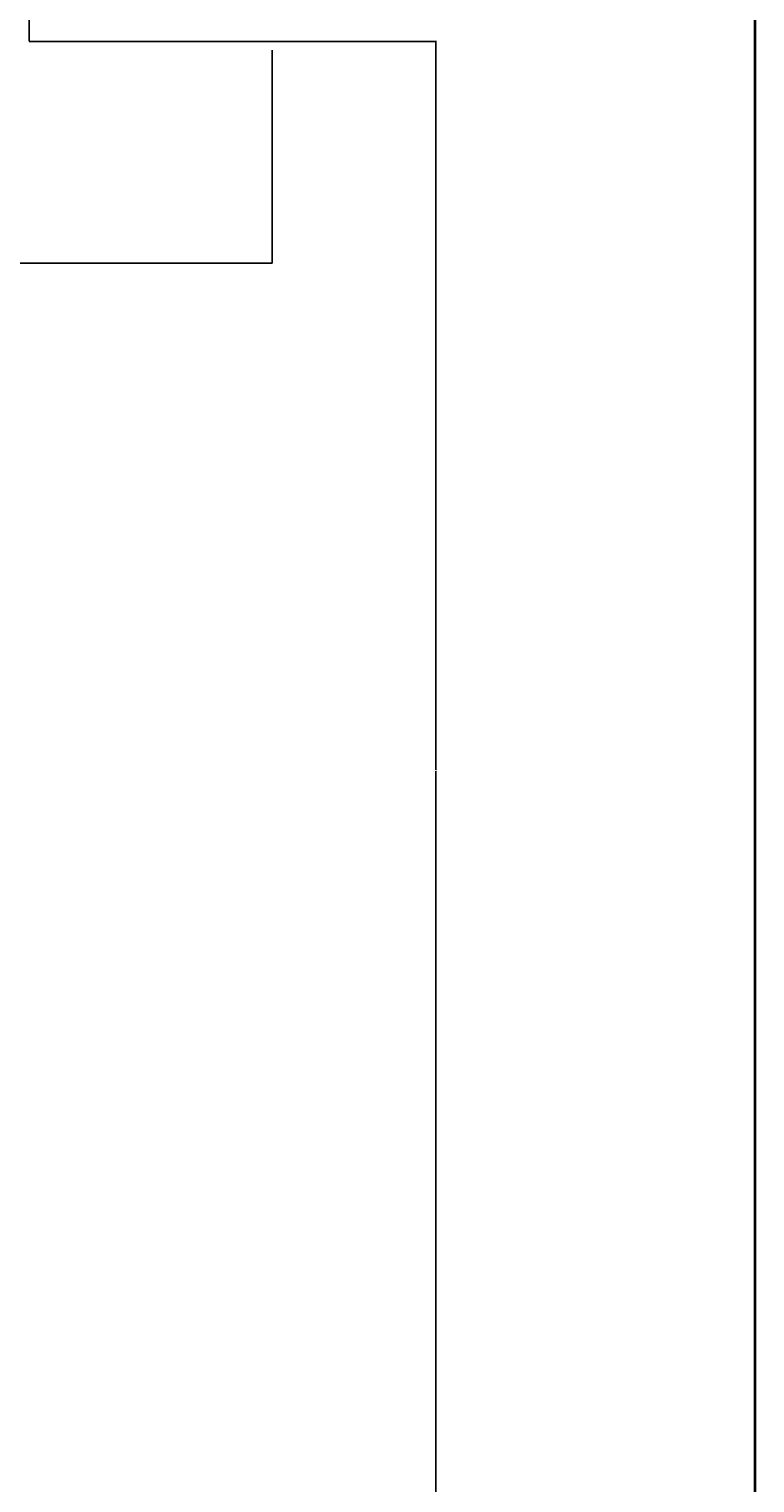
# Model space of a CAD drawing. Units: inches. Extents: x 2120 to 4013, y 1390 to 3019.
# Tile 54 of 59: x 3819 to 4013, y 1967 to 2356. Entities that reach past the tile are written whole.
import ezdxf

# ---------------------------------------------------------------- set-up
doc = ezdxf.new("R2010")
doc.units = ezdxf.units.IN
for name, color, linetype, lineweight in [('A-ANNO-DIMS', 2, 'Continuous', 18), ('A-ANNO-SYMB', 2, 'Continuous', 25), ('A-ANNO-TTLB', 7, 'Continuous', 35), ('A-WALL-PATT', 252, 'Continuous', 13)]:
    doc.layers.add(name, color=color, linetype=linetype, lineweight=lineweight)
doc.styles.get("Standard").update_dxf_attribs({"font": 'arial.ttf'})
doc.dimstyles.get("Standard").update_dxf_attribs({"dimtxt": 0.18, "dimasz": 0.18, "dimexe": 0.18, "dimexo": 0.0625, "dimgap": 0.09, "dimtad": 0, "dimtih": 1, "dimtoh": 1, "dimdec": 4, "dimzin": 0, "dimdsep": 46, "dimtxsty": 'Standard', "dimcen": 0.09, "dimadec": 0, "dimazin": 0, "dimtfac": 1, "dimtdec": 4, "dimtofl": 0, "dimtmove": 0, "dimatfit": 3, "dimfxl": 1, "dimtolj": 1, "dimtzin": 0, "dimarcsym": 0})

# ---------------------------------------------------------------- blocks, each defined once
blk = doc.blocks.new('*D216')
at = {"layer": 'A-ANNO-DIMS', "color": 0, "lineweight": -2, "transparency": 16777216}
for p, q in [((3071.73, 2352.59), (3071.73, 2396.46)), ((3071.91, 2396.28), (3444.95, 2396.28)), ((3818.55, 2396.28), (3445.52, 2396.28)), ((3818.73, 2352.59), (3818.73, 2396.46))]:
    blk.add_line(p, q, dxfattribs=at)
at = {"layer": 'A-ANNO-DIMS', "color": 0, "transparency": 16777216}
for points in [[(3071.91, 2396.31), (3071.91, 2396.25), (3071.73, 2396.28)], [(3818.55, 2396.31), (3818.55, 2396.25), (3818.73, 2396.28)]]:
    blk.add_solid(points, dxfattribs=at)
at = {"layer": 'Defpoints', "color": 0, "transparency": 16777216}
for p in [(3818.73, 2396.28), (3071.73, 2352.53), (3818.73, 2352.53)]:
    blk.add_point(p, dxfattribs=at)
at = {"layer": 'A-ANNO-DIMS', "color": 0, "transparency": 16777216, "insert": (3445.23, 2396.28), "char_height": 0.18, "attachment_point": 5}
blk.add_mtext('\\A1;747', dxfattribs=at)
blk = doc.blocks.new('*D218')
at = {"layer": 'A-ANNO-DIMS', "color": 0, "lineweight": -2, "transparency": 16777216}
for p, q in [((3818.8, 2352.53), (3927.73, 2352.53)), ((3927.55, 2352.35), (3927.55, 2157.71)), ((3927.55, 1962.71), (3927.55, 2157.35)), ((3818.8, 1962.53), (3927.73, 1962.53))]:
    blk.add_line(p, q, dxfattribs=at)
at = {"layer": 'A-ANNO-DIMS', "color": 0, "transparency": 16777216}
for points in [[(3927.52, 2352.35), (3927.58, 2352.35), (3927.55, 2352.53)], [(3927.52, 1962.71), (3927.58, 1962.71), (3927.55, 1962.53)]]:
    blk.add_solid(points, dxfattribs=at)
at = {"layer": 'Defpoints', "color": 0, "transparency": 16777216}
for p in [(3818.73, 2352.53), (3818.73, 1962.53), (3927.55, 1962.53)]:
    blk.add_point(p, dxfattribs=at)
at = {"layer": 'A-ANNO-DIMS', "color": 0, "transparency": 16777216, "insert": (3927.55, 2157.53), "char_height": 0.18, "attachment_point": 5}
blk.add_mtext('\\A1;390', dxfattribs=at)

msp = doc.modelspace()

# ---------------------------------------------------------------- hatches: boundary and pattern name
at = {"layer": 'A-WALL-PATT'}
h = msp.add_hatch(dxfattribs=at)
h.set_pattern_fill('ANSI32', color=256)
h.paths.add_polyline_path([(2271.7331, 2343.531), (2283.3788, 2343.531), (2283.3788, 2348.031), (2283.3788, 2352.5306), (2262.7331, 2352.5306), (2262.7331, 2182.638), (2267.2331, 2182.638), (2271.7331, 2182.638), (2271.7331, 2219.031), (2391.7331, 2219.031), (2391.7331, 2214.189), (2393.9831, 2214.189), (2396.2331, 2214.189), (2396.2331, 2219.031), (2420.2331, 2219.031), (2420.2331, 2225.7535), (2417.2197, 2225.7535), (2415.7331, 2225.7535), (2415.7331, 2223.5306), (2271.7331, 2223.5306)])
h.paths.add_polyline_path([(2380.0942, 2352.5306), (2343.3788, 2352.5306), (2343.3788, 2343.531), (2363.2331, 2343.531), (2363.2331, 2288.8489), (2365.4831, 2288.8489), (2367.7331, 2288.8489), (2367.7331, 2343.531), (2380.0942, 2343.531)], flags=17)
h.paths.add_polyline_path([(2432.4339, 2352.5306), (2404.0943, 2352.5306), (2404.0943, 2343.531), (2415.7331, 2343.531), (2415.7331, 2264.0306), (2367.7331, 2264.0306), (2367.7331, 2266.4872), (2363.2331, 2266.4872), (2363.2331, 2259.531), (2367.7331, 2259.531), (2415.7331, 2259.531), (2415.7331, 2255.0658), (2420.2331, 2255.0658), (2420.2331, 2259.531), (2424.5717, 2259.531), (2424.5717, 2261.781), (2424.5717, 2264.0306), (2420.2331, 2264.0306), (2420.2331, 2343.531), (2432.4339, 2343.531)])
h.paths.add_polyline_path([(2508.9115, 2352.5306), (2456.4339, 2352.5306), (2456.4339, 2343.531), (2468.2331, 2343.531), (2468.2331, 2264.0306), (2448.0487, 2264.0306), (2448.0487, 2259.531), (2468.2331, 2259.531), (2468.2331, 2255.5496), (2472.7331, 2255.5496), (2472.7331, 2343.531), (2508.9115, 2343.531)])
h.paths.add_polyline_path([(2637.7331, 2352.5306), (2544.9116, 2352.5306), (2544.9116, 2343.531), (2589.7331, 2343.531), (2633.2331, 2343.531), (2637.7331, 2343.531)])
h.paths.add_polyline_path([(2594.2331, 2343.5306), (2589.7331, 2343.5306), (2589.7331, 2259.5306), (2589.7331, 2252.4915), (2591.9831, 2252.4915), (2594.2331, 2252.4915)])
h.paths.add_polyline_path([(2637.7331, 2223.5306), (2594.2331, 2223.5306), (2594.2331, 2230.1988), (2591.9831, 2230.1988), (2589.7331, 2230.1988), (2589.7331, 2223.5306), (2472.7331, 2223.5306), (2468.2331, 2223.5306), (2468.2331, 2219.031), (2628.7331, 2219.031), (2628.7331, 2138.031), (2637.7331, 2138.031)])
h.paths.add_polyline_path([(3822.6535, 2458.4402), (3874.9468, 2458.4402), (3874.9468, 2476.9866), (3822.6535, 2476.9866)], flags=9)
h.paths.add_polyline_path([(3834.6921, 2781.8174), (3935.9206, 2781.8174), (3935.9206, 2800.3638), (3834.6921, 2800.3638)], flags=9)
h.paths.add_polyline_path([(3832.2843, 2837.9683), (3884.5776, 2837.9683), (3884.5776, 2856.5146), (3832.2843, 2856.5146)], flags=9)
h.paths.add_polyline_path([(3830.9388, 2861.4782), (3956.8958, 2861.4782), (3956.8958, 2880.0245), (3830.9388, 2880.0245)], flags=9)
h.paths.add_polyline_path([(3870.6966, 2352.5752), (3887.9272, 2352.5752), (3887.9272, 2377.3037), (3870.6966, 2377.3037)], flags=9)
h.paths.add_polyline_path([(3289.2701, 2413.161), (3435.2223, 2413.161), (3435.2223, 2450.2538), (3289.2701, 2450.2538)], flags=9)
h.paths.add_polyline_path([(2487.6944, 2414.3601), (2637.8335, 2414.3601), (2637.8335, 2451.4528), (2487.6944, 2451.4528)], flags=9)
h.paths.add_polyline_path([(2567.3724, 1457.9199), (2815.296, 1457.9199), (2815.296, 1495.0127), (2567.3724, 1495.0127)], flags=9)
h.paths.add_polyline_path([(2655.3825, 2093.2363), (2685.9555, 2093.2363), (2685.9555, 2111.8937), (2655.3825, 2111.8937)], flags=9)
h.paths.add_polyline_path([(2543.9218, 1550.6671), (2587.8406, 1550.6671), (2587.8406, 1569.3244), (2543.9218, 1569.3244)], flags=9)
h.paths.add_polyline_path([(2905.1384, 1543.8113), (2949.0572, 1543.8113), (2949.0572, 1562.4686), (2905.1384, 1562.4686)], flags=9)
h.paths.add_polyline_path([(2736.4118, 1702.4736), (2784.2153, 1702.4736), (2784.2153, 1721.1309), (2736.4118, 1721.1309)], flags=9)
h.paths.add_polyline_path([(2912.8666, 1710.4168), (2951.707, 1710.4168), (2951.707, 1729.0741), (2912.8666, 1729.0741)], flags=9)
h.paths.add_polyline_path([(2923.5785, 1763.5038), (2959.7279, 1763.5038), (2959.7279, 1782.1611), (2923.5785, 1782.1611)], flags=9)
h.paths.add_polyline_path([(2925.2114, 1809.6137), (2967.1861, 1809.6137), (2967.1861, 1828.271), (2925.2114, 1828.271)], flags=9)
h.paths.add_polyline_path([(2996.2711, 1878.9003), (2996.2711, 1913.109), (2977.6138, 1913.109), (2977.6138, 1878.9003)], flags=9)
h.paths.add_polyline_path([(2883.0859, 1895.7192), (2927.1855, 1895.7192), (2927.1855, 1914.3766), (2883.0859, 1914.3766)], flags=9)
h.paths.add_polyline_path([(2787.3924, 1810.8013), (2841.0213, 1810.8013), (2841.0213, 1829.4587), (2787.3924, 1829.4587)], flags=9)
h.paths.add_polyline_path([(2775.6399, 2101.7395), (2829.2689, 2101.7395), (2829.2689, 2120.3968), (2775.6399, 2120.3968)], flags=9)
h.paths.add_polyline_path([(2913.0263, 2075.817), (2951.8667, 2075.817), (2951.8667, 2094.4744), (2913.0263, 2094.4744)], flags=9)
h.paths.add_polyline_path([(2929.966, 2133.3669), (2966.1154, 2133.3669), (2966.1154, 2152.0243), (2929.966, 2152.0243)], flags=9)
h.paths.add_polyline_path([(2932.7502, 2182.6088), (2968.8996, 2182.6088), (2968.8996, 2201.2662), (2932.7502, 2201.2662)], flags=9)
h.paths.add_polyline_path([(2996.0681, 2266.3173), (2996.0681, 2300.5261), (2977.4108, 2300.5261), (2977.4108, 2266.3173)], flags=9)
h.paths.add_polyline_path([(2885.1039, 2279.2186), (2929.2035, 2279.2186), (2929.2035, 2297.8759), (2885.1039, 2297.8759)], flags=9)
h.paths.add_polyline_path([(2735.7042, 2218.3197), (2783.5078, 2218.3197), (2783.5078, 2236.9771), (2735.7042, 2236.9771)], flags=9)
h.paths.add_polyline_path([(2635.6049, 2044.0085), (2648.9678, 2044.0085), (2648.9678, 2054.312), (2635.6049, 2054.312)], flags=9)
h.paths.add_polyline_path([(2714.0148, 1923.0473), (2727.3777, 1923.0473), (2727.3777, 1933.3508), (2714.0148, 1933.3508)], flags=9)
h.paths.add_polyline_path([(2709.0345, 1988.1628), (2722.3974, 1988.1628), (2722.3974, 1998.4663), (2709.0345, 1998.4663)], flags=9)
h.paths.add_polyline_path([(2592.8935, 1962.1763), (2606.2564, 1962.1763), (2606.2564, 1972.4799), (2592.8935, 1972.4799)], flags=9)
h.paths.add_polyline_path([(2618.3996, 1985.9724), (2644.1942, 1985.9724), (2644.1942, 1996.2759), (2618.3996, 1996.2759)], flags=9)
h.paths.add_polyline_path([(2601.279, 1920.5869), (2614.6419, 1920.5869), (2614.6419, 1930.8904), (2601.279, 1930.8904)], flags=9)
h.paths.add_polyline_path([(2692.3278, 1932.7645), (2704.5311, 1932.7645), (2704.5311, 1943.0681), (2692.3278, 1943.0681)], flags=9)
h.paths.add_polyline_path([(2311.122, 1672.7318), (2355.0408, 1672.7318), (2355.0408, 1691.3892), (2311.122, 1691.3892)], flags=9)
h.paths.add_polyline_path([(2456.2551, 1632.3198), (2492.4796, 1632.3198), (2492.4796, 1650.9772), (2456.2551, 1650.9772)], flags=9)
h.paths.add_polyline_path([(2401.0766, 1631.4793), (2437.301, 1631.4793), (2437.301, 1650.1367), (2401.0766, 1650.1367)], flags=9)
h.paths.add_polyline_path([(2546.7054, 1700.9235), (2594.509, 1700.9235), (2594.509, 1719.5809), (2546.7054, 1719.5809)], flags=9)
h.paths.add_polyline_path([(2445.4866, 1766.9937), (2497.5261, 1766.9937), (2497.5261, 1785.651), (2445.4866, 1785.651)], flags=9)
h.paths.add_polyline_path([(2287.9992, 1739.7675), (2326.8396, 1739.7675), (2326.8396, 1758.4248), (2287.9992, 1758.4248)], flags=9)
h.paths.add_polyline_path([(2458.5279, 1924.7607), (2510.5675, 1924.7607), (2510.5675, 1943.4181), (2458.5279, 1943.4181)], flags=9)
h.paths.add_polyline_path([(2309.2811, 1902.7642), (2345.4305, 1902.7642), (2345.4305, 1921.4215), (2309.2811, 1921.4215)], flags=9)
h.paths.add_polyline_path([(2490.7554, 2018.9392), (2530.7896, 2018.9392), (2530.7896, 2037.5965), (2490.7554, 2037.5965)], flags=9)
h.paths.add_polyline_path([(2402.143, 2024.7393), (2438.5414, 2024.7393), (2438.5414, 2043.3966), (2402.143, 2043.3966)], flags=9)
h.paths.add_polyline_path([(2287.856, 1931.7926), (2326.6964, 1931.7926), (2326.6964, 1950.4499), (2287.856, 1950.4499)], flags=9)
h.paths.add_polyline_path([(2281.7979, 2193.5771), (2320.6383, 2193.5771), (2320.6383, 2212.2344), (2281.7979, 2212.2344)], flags=25)
h.paths.add_polyline_path([(2484.0754, 2093.892), (2536.115, 2093.892), (2536.115, 2112.5494), (2484.0754, 2112.5494)], flags=9)
h.paths.add_polyline_path([(2624.7948, 2281.8639), (2624.7948, 2311.4137), (2606.1375, 2311.4137), (2606.1375, 2281.8639)], flags=9)
h.paths.add_polyline_path([(2507.5036, 2290.3639), (2541.934, 2290.3639), (2541.934, 2309.0212), (2507.5036, 2309.0212)], flags=9)
h.paths.add_polyline_path([(2423.1076, 2285.2202), (2459.332, 2285.2202), (2459.332, 2303.8776), (2423.1076, 2303.8776)], flags=9)
h.paths.add_polyline_path([(2374.5467, 2289.6272), (2410.7711, 2289.6272), (2410.7711, 2308.2846), (2374.5467, 2308.2846)], flags=25)
h.paths.add_polyline_path([(2277.4907, 2227.5651), (2316.3311, 2227.5651), (2316.3311, 2246.2224), (2277.4907, 2246.2224)], flags=25)
h.paths.add_polyline_path([(2655.3825, 2093.2367), (2685.9555, 2093.2367), (2685.9555, 2111.894), (2655.3825, 2111.894)], flags=9)
h.paths.add_polyline_path([(2543.9217, 1550.6674), (2587.8406, 1550.6674), (2587.8406, 1569.3247), (2543.9217, 1569.3247)], flags=9)
h.paths.add_polyline_path([(2905.1384, 1543.8116), (2949.0572, 1543.8116), (2949.0572, 1562.4689), (2905.1384, 1562.4689)], flags=9)
h.paths.add_polyline_path([(2736.4118, 1702.4739), (2784.2153, 1702.4739), (2784.2153, 1721.1312), (2736.4118, 1721.1312)], flags=9)
h.paths.add_polyline_path([(2912.8666, 1710.4171), (2951.707, 1710.4171), (2951.707, 1729.0744), (2912.8666, 1729.0744)], flags=9)
h.paths.add_polyline_path([(2923.5785, 1763.5041), (2959.7279, 1763.5041), (2959.7279, 1782.1614), (2923.5785, 1782.1614)], flags=9)
h.paths.add_polyline_path([(2925.2114, 1809.614), (2967.1861, 1809.614), (2967.1861, 1828.2713), (2925.2114, 1828.2713)], flags=9)
h.paths.add_polyline_path([(2996.2711, 1878.9006), (2996.2711, 1913.1094), (2977.6137, 1913.1094), (2977.6137, 1878.9006)], flags=9)
h.paths.add_polyline_path([(2883.0859, 1895.7195), (2927.1855, 1895.7195), (2927.1855, 1914.3769), (2883.0859, 1914.3769)], flags=9)
h.paths.add_polyline_path([(2787.3924, 1810.8016), (2841.0213, 1810.8016), (2841.0213, 1829.459), (2787.3924, 1829.459)], flags=9)
h.paths.add_polyline_path([(2775.6399, 2101.7398), (2829.2688, 2101.7398), (2829.2688, 2120.3971), (2775.6399, 2120.3971)], flags=9)
h.paths.add_polyline_path([(2913.0263, 2075.8173), (2951.8667, 2075.8173), (2951.8667, 2094.4747), (2913.0263, 2094.4747)], flags=9)
h.paths.add_polyline_path([(2929.966, 2133.3672), (2966.1154, 2133.3672), (2966.1154, 2152.0246), (2929.966, 2152.0246)], flags=9)
h.paths.add_polyline_path([(2932.7502, 2182.6091), (2968.8996, 2182.6091), (2968.8996, 2201.2665), (2932.7502, 2201.2665)], flags=9)
h.paths.add_polyline_path([(2996.0681, 2266.3176), (2996.0681, 2300.5264), (2977.4108, 2300.5264), (2977.4108, 2266.3176)], flags=9)
h.paths.add_polyline_path([(2885.1039, 2279.2189), (2929.2035, 2279.2189), (2929.2035, 2297.8762), (2885.1039, 2297.8762)], flags=9)
h.paths.add_polyline_path([(2735.7042, 2218.32), (2783.5078, 2218.32), (2783.5078, 2236.9774), (2735.7042, 2236.9774)], flags=9)
h.paths.add_polyline_path([(2635.6048, 2044.0088), (2648.9677, 2044.0088), (2648.9677, 2054.3123), (2635.6048, 2054.3123)], flags=9)
h.paths.add_polyline_path([(2714.0148, 1923.0476), (2727.3777, 1923.0476), (2727.3777, 1933.3511), (2714.0148, 1933.3511)], flags=9)
h.paths.add_polyline_path([(2709.0345, 1988.1631), (2722.3974, 1988.1631), (2722.3974, 1998.4666), (2709.0345, 1998.4666)], flags=9)
h.paths.add_polyline_path([(2592.8935, 1962.1766), (2606.2564, 1962.1766), (2606.2564, 1972.4802), (2592.8935, 1972.4802)], flags=9)
h.paths.add_polyline_path([(2618.3995, 1985.9727), (2644.1942, 1985.9727), (2644.1942, 1996.2762), (2618.3995, 1996.2762)], flags=9)
h.paths.add_polyline_path([(2601.279, 1920.5872), (2614.6419, 1920.5872), (2614.6419, 1930.8908), (2601.279, 1930.8908)], flags=9)
h.paths.add_polyline_path([(2692.3278, 1932.7648), (2704.5311, 1932.7648), (2704.5311, 1943.0684), (2692.3278, 1943.0684)], flags=9)
h.paths.add_polyline_path([(2311.122, 1672.7321), (2355.0408, 1672.7321), (2355.0408, 1691.3895), (2311.122, 1691.3895)], flags=9)
h.paths.add_polyline_path([(2456.2551, 1632.3201), (2492.4795, 1632.3201), (2492.4795, 1650.9775), (2456.2551, 1650.9775)], flags=9)
h.paths.add_polyline_path([(2401.0766, 1631.4796), (2437.301, 1631.4796), (2437.301, 1650.137), (2401.0766, 1650.137)], flags=9)
h.paths.add_polyline_path([(2546.7054, 1700.9238), (2594.509, 1700.9238), (2594.509, 1719.5812), (2546.7054, 1719.5812)], flags=9)
h.paths.add_polyline_path([(2445.4866, 1766.994), (2497.5261, 1766.994), (2497.5261, 1785.6513), (2445.4866, 1785.6513)], flags=9)
h.paths.add_polyline_path([(2287.9992, 1739.7678), (2326.8396, 1739.7678), (2326.8396, 1758.4251), (2287.9992, 1758.4251)], flags=9)
h.paths.add_polyline_path([(2458.5279, 1924.7611), (2510.5675, 1924.7611), (2510.5675, 1943.4184), (2458.5279, 1943.4184)], flags=9)
h.paths.add_polyline_path([(2309.2811, 1902.7645), (2345.4305, 1902.7645), (2345.4305, 1921.4218), (2309.2811, 1921.4218)], flags=9)
h.paths.add_polyline_path([(2490.7554, 2018.9395), (2530.7895, 2018.9395), (2530.7895, 2037.5968), (2490.7554, 2037.5968)], flags=9)
h.paths.add_polyline_path([(2402.143, 2024.7396), (2438.5413, 2024.7396), (2438.5413, 2043.3969), (2402.143, 2043.3969)], flags=9)
h.paths.add_polyline_path([(2287.856, 1931.7929), (2326.6964, 1931.7929), (2326.6964, 1950.4502), (2287.856, 1950.4502)], flags=9)
h.paths.add_polyline_path([(2281.7979, 2193.5774), (2320.6383, 2193.5774), (2320.6383, 2212.2347), (2281.7979, 2212.2347)], flags=25)
h.paths.add_polyline_path([(2484.0754, 2093.8924), (2536.115, 2093.8924), (2536.115, 2112.5497), (2484.0754, 2112.5497)], flags=9)
h.paths.add_polyline_path([(2624.7948, 2281.8642), (2624.7948, 2311.414), (2606.1374, 2311.414), (2606.1374, 2281.8642)], flags=9)
h.paths.add_polyline_path([(2507.5035, 2290.3642), (2541.934, 2290.3642), (2541.934, 2309.0215), (2507.5035, 2309.0215)], flags=9)
h.paths.add_polyline_path([(2423.1075, 2285.2205), (2459.332, 2285.2205), (2459.332, 2303.8779), (2423.1075, 2303.8779)], flags=9)
h.paths.add_polyline_path([(2374.5467, 2289.6275), (2410.7711, 2289.6275), (2410.7711, 2308.2849), (2374.5467, 2308.2849)], flags=25)
h.paths.add_polyline_path([(2277.4907, 2227.5654), (2316.3311, 2227.5654), (2316.3311, 2246.2227), (2277.4907, 2246.2227)], flags=25)
h = msp.add_hatch(dxfattribs=at)
h.set_pattern_fill('ANSI32', color=256)
h.paths.add_polyline_path([(2271.7331, 1980.389), (2262.7331, 1980.389), (2262.7331, 1912.8434), (2267.2331, 1912.8434), (2271.7331, 1912.8434), (2271.7331, 1922.531), (2351.2331, 1922.531), (2351.2331, 1901.4728), (2355.7331, 1901.4728), (2355.7331, 1922.531), (2357.9815, 1922.531), (2357.9815, 1926.5306), (2271.7331, 1926.5306)])
h.paths.add_polyline_path([(2589.2331, 1949.1622), (2584.7331, 1949.1622), (2580.2331, 1949.1622), (2580.2331, 1874.5306), (2355.7331, 1874.5306), (2355.7331, 1880.1922), (2351.2331, 1880.1922), (2351.2331, 1874.5306), (2271.7331, 1874.5306), (2271.7331, 1888.8431), (2262.7331, 1888.8431), (2262.7331, 1842.2909), (2267.2331, 1842.2909), (2271.7331, 1842.2909), (2271.7331, 1865.531), (2415.7331, 1865.531), (2415.7331, 1779.7286), (2420.2331, 1779.7286), (2420.2331, 1865.531), (2589.2331, 1865.531)])
h.paths.add_polyline_path([(2271.7331, 1782.2906), (2262.7331, 1782.2906), (2262.7331, 1711.4639), (2267.2331, 1711.4639), (2271.7331, 1711.4639), (2271.7331, 1738.031), (2420.2331, 1738.031), (2420.2331, 1742.531), (2420.2331, 1747.3376), (2417.9831, 1747.3376), (2415.7331, 1747.3376), (2415.7331, 1742.5306), (2271.7331, 1742.5306)])
h.paths.add_polyline_path([(2271.7331, 1627.031), (2362.3957, 1627.031), (2362.3957, 1629.281), (2362.3957, 1631.5306), (2271.7331, 1631.5306), (2271.7331, 1675.4636), (2262.7331, 1675.4636), (2262.7331, 1581.531), (2405.3032, 1581.531), (2405.3032, 1586.031), (2405.3032, 1590.5306), (2396.2331, 1590.5306), (2396.2331, 1691.4513), (2418.7206, 1691.4513), (2418.7206, 1695.951), (2396.2331, 1695.951), (2391.7331, 1695.951), (2391.7331, 1631.5306), (2386.7425, 1631.5306), (2386.7425, 1629.2806), (2386.7425, 1627.031), (2391.7331, 1627.031), (2391.7331, 1586.1709), (2271.7331, 1586.1709)])
h.paths.add_polyline_path([(2459.6703, 1590.5306), (2429.3032, 1590.5306), (2429.3032, 1581.531), (2459.6703, 1581.531), (2459.6703, 1586.031)])
h.paths.add_polyline_path([(2501.2331, 1590.531), (2501.2331, 1665.0195), (2498.9831, 1665.0195), (2496.7331, 1665.0195), (2496.7331, 1590.5306), (2483.8201, 1590.5306), (2483.8201, 1590.1579), (2483.6704, 1590.1579), (2483.6704, 1581.531), (2505.0196, 1581.531), (2505.0196, 1583.781), (2505.0196, 1586.0306), (2501.2331, 1586.0306)])
h.paths.add_polyline_path([(2544.1361, 1583.781), (2544.1361, 1586.0306), (2527.1368, 1586.0306), (2527.1368, 1583.7806), (2527.1368, 1581.531), (2544.1361, 1581.531)])
h.paths.add_polyline_path([(3822.6535, 2458.4402), (3874.9468, 2458.4402), (3874.9468, 2476.9866), (3822.6535, 2476.9866)], flags=9)
h.paths.add_polyline_path([(3834.6921, 2781.8174), (3935.9206, 2781.8174), (3935.9206, 2800.3638), (3834.6921, 2800.3638)], flags=9)
h.paths.add_polyline_path([(3832.2843, 2837.9683), (3884.5776, 2837.9683), (3884.5776, 2856.5146), (3832.2843, 2856.5146)], flags=9)
h.paths.add_polyline_path([(3830.9388, 2861.4782), (3956.8958, 2861.4782), (3956.8958, 2880.0245), (3830.9388, 2880.0245)], flags=9)
h.paths.add_polyline_path([(3870.6966, 2352.5752), (3887.9272, 2352.5752), (3887.9272, 2377.3037), (3870.6966, 2377.3037)], flags=9)
h.paths.add_polyline_path([(3289.2701, 2413.161), (3435.2223, 2413.161), (3435.2223, 2450.2538), (3289.2701, 2450.2538)], flags=9)
h.paths.add_polyline_path([(2487.6944, 2414.3601), (2637.8335, 2414.3601), (2637.8335, 2451.4528), (2487.6944, 2451.4528)], flags=9)
h.paths.add_polyline_path([(2567.3724, 1457.9199), (2815.296, 1457.9199), (2815.296, 1495.0127), (2567.3724, 1495.0127)], flags=9)
h.paths.add_polyline_path([(2655.3825, 2093.2363), (2685.9555, 2093.2363), (2685.9555, 2111.8937), (2655.3825, 2111.8937)], flags=9)
h.paths.add_polyline_path([(2543.9218, 1550.6671), (2587.8406, 1550.6671), (2587.8406, 1569.3244), (2543.9218, 1569.3244)], flags=9)
h.paths.add_polyline_path([(2905.1384, 1543.8113), (2949.0572, 1543.8113), (2949.0572, 1562.4686), (2905.1384, 1562.4686)], flags=9)
h.paths.add_polyline_path([(2736.4118, 1702.4736), (2784.2153, 1702.4736), (2784.2153, 1721.1309), (2736.4118, 1721.1309)], flags=9)
h.paths.add_polyline_path([(2912.8666, 1710.4168), (2951.707, 1710.4168), (2951.707, 1729.0741), (2912.8666, 1729.0741)], flags=9)
h.paths.add_polyline_path([(2923.5785, 1763.5038), (2959.7279, 1763.5038), (2959.7279, 1782.1611), (2923.5785, 1782.1611)], flags=9)
h.paths.add_polyline_path([(2925.2114, 1809.6137), (2967.1861, 1809.6137), (2967.1861, 1828.271), (2925.2114, 1828.271)], flags=9)
h.paths.add_polyline_path([(2996.2711, 1878.9003), (2996.2711, 1913.109), (2977.6138, 1913.109), (2977.6138, 1878.9003)], flags=9)
h.paths.add_polyline_path([(2883.0859, 1895.7192), (2927.1855, 1895.7192), (2927.1855, 1914.3766), (2883.0859, 1914.3766)], flags=9)
h.paths.add_polyline_path([(2787.3924, 1810.8013), (2841.0213, 1810.8013), (2841.0213, 1829.4587), (2787.3924, 1829.4587)], flags=9)
h.paths.add_polyline_path([(2775.6399, 2101.7395), (2829.2689, 2101.7395), (2829.2689, 2120.3968), (2775.6399, 2120.3968)], flags=9)
h.paths.add_polyline_path([(2913.0263, 2075.817), (2951.8667, 2075.817), (2951.8667, 2094.4744), (2913.0263, 2094.4744)], flags=9)
h.paths.add_polyline_path([(2929.966, 2133.3669), (2966.1154, 2133.3669), (2966.1154, 2152.0243), (2929.966, 2152.0243)], flags=9)
h.paths.add_polyline_path([(2932.7502, 2182.6088), (2968.8996, 2182.6088), (2968.8996, 2201.2662), (2932.7502, 2201.2662)], flags=9)
h.paths.add_polyline_path([(2996.0681, 2266.3173), (2996.0681, 2300.5261), (2977.4108, 2300.5261), (2977.4108, 2266.3173)], flags=9)
h.paths.add_polyline_path([(2885.1039, 2279.2186), (2929.2035, 2279.2186), (2929.2035, 2297.8759), (2885.1039, 2297.8759)], flags=9)
h.paths.add_polyline_path([(2735.7042, 2218.3197), (2783.5078, 2218.3197), (2783.5078, 2236.9771), (2735.7042, 2236.9771)], flags=9)
h.paths.add_polyline_path([(2635.6049, 2044.0085), (2648.9678, 2044.0085), (2648.9678, 2054.312), (2635.6049, 2054.312)], flags=9)
h.paths.add_polyline_path([(2714.0148, 1923.0473), (2727.3777, 1923.0473), (2727.3777, 1933.3508), (2714.0148, 1933.3508)], flags=9)
h.paths.add_polyline_path([(2709.0345, 1988.1628), (2722.3974, 1988.1628), (2722.3974, 1998.4663), (2709.0345, 1998.4663)], flags=9)
h.paths.add_polyline_path([(2592.8935, 1962.1763), (2606.2564, 1962.1763), (2606.2564, 1972.4799), (2592.8935, 1972.4799)], flags=9)
h.paths.add_polyline_path([(2618.3996, 1985.9724), (2644.1942, 1985.9724), (2644.1942, 1996.2759), (2618.3996, 1996.2759)], flags=9)
h.paths.add_polyline_path([(2601.279, 1920.5869), (2614.6419, 1920.5869), (2614.6419, 1930.8904), (2601.279, 1930.8904)], flags=9)
h.paths.add_polyline_path([(2692.3278, 1932.7645), (2704.5311, 1932.7645), (2704.5311, 1943.0681), (2692.3278, 1943.0681)], flags=9)
h.paths.add_polyline_path([(2311.122, 1672.7318), (2355.0408, 1672.7318), (2355.0408, 1691.3892), (2311.122, 1691.3892)], flags=25)
h.paths.add_polyline_path([(2456.2551, 1632.3198), (2492.4796, 1632.3198), (2492.4796, 1650.9772), (2456.2551, 1650.9772)], flags=9)
h.paths.add_polyline_path([(2401.0766, 1631.4793), (2437.301, 1631.4793), (2437.301, 1650.1367), (2401.0766, 1650.1367)], flags=9)
h.paths.add_polyline_path([(2546.7054, 1700.9235), (2594.509, 1700.9235), (2594.509, 1719.5809), (2546.7054, 1719.5809)], flags=9)
h.paths.add_polyline_path([(2445.4866, 1766.9937), (2497.5261, 1766.9937), (2497.5261, 1785.651), (2445.4866, 1785.651)], flags=9)
h.paths.add_polyline_path([(2287.9992, 1739.7675), (2326.8396, 1739.7675), (2326.8396, 1758.4248), (2287.9992, 1758.4248)], flags=24)
h.paths.add_polyline_path([(2458.5279, 1924.7607), (2510.5675, 1924.7607), (2510.5675, 1943.4181), (2458.5279, 1943.4181)], flags=25)
h.paths.add_polyline_path([(2309.2811, 1902.7642), (2345.4305, 1902.7642), (2345.4305, 1921.4215), (2309.2811, 1921.4215)], flags=25)
h.paths.add_polyline_path([(2490.7554, 2018.9392), (2530.7896, 2018.9392), (2530.7896, 2037.5965), (2490.7554, 2037.5965)], flags=9)
h.paths.add_polyline_path([(2402.143, 2024.7393), (2438.5414, 2024.7393), (2438.5414, 2043.3966), (2402.143, 2043.3966)], flags=9)
h.paths.add_polyline_path([(2287.856, 1931.7926), (2326.6964, 1931.7926), (2326.6964, 1950.4499), (2287.856, 1950.4499)], flags=25)
h.paths.add_polyline_path([(2281.7979, 2193.5771), (2320.6383, 2193.5771), (2320.6383, 2212.2344), (2281.7979, 2212.2344)], flags=9)
h.paths.add_polyline_path([(2484.0754, 2093.892), (2536.115, 2093.892), (2536.115, 2112.5494), (2484.0754, 2112.5494)], flags=9)
h.paths.add_polyline_path([(2624.7948, 2281.8639), (2624.7948, 2311.4137), (2606.1375, 2311.4137), (2606.1375, 2281.8639)], flags=9)
h.paths.add_polyline_path([(2507.5036, 2290.3639), (2541.934, 2290.3639), (2541.934, 2309.0212), (2507.5036, 2309.0212)], flags=9)
h.paths.add_polyline_path([(2423.1076, 2285.2202), (2459.332, 2285.2202), (2459.332, 2303.8776), (2423.1076, 2303.8776)], flags=9)
h.paths.add_polyline_path([(2374.5467, 2289.6272), (2410.7711, 2289.6272), (2410.7711, 2308.2846), (2374.5467, 2308.2846)], flags=9)
h.paths.add_polyline_path([(2277.4907, 2227.5651), (2316.3311, 2227.5651), (2316.3311, 2246.2224), (2277.4907, 2246.2224)], flags=9)
h.paths.add_polyline_path([(2655.3825, 2093.2367), (2685.9555, 2093.2367), (2685.9555, 2111.894), (2655.3825, 2111.894)], flags=9)
h.paths.add_polyline_path([(2543.9217, 1550.6674), (2587.8406, 1550.6674), (2587.8406, 1569.3247), (2543.9217, 1569.3247)], flags=9)
h.paths.add_polyline_path([(2905.1384, 1543.8116), (2949.0572, 1543.8116), (2949.0572, 1562.4689), (2905.1384, 1562.4689)], flags=9)
h.paths.add_polyline_path([(2736.4118, 1702.4739), (2784.2153, 1702.4739), (2784.2153, 1721.1312), (2736.4118, 1721.1312)], flags=9)
h.paths.add_polyline_path([(2912.8666, 1710.4171), (2951.707, 1710.4171), (2951.707, 1729.0744), (2912.8666, 1729.0744)], flags=9)
h.paths.add_polyline_path([(2923.5785, 1763.5041), (2959.7279, 1763.5041), (2959.7279, 1782.1614), (2923.5785, 1782.1614)], flags=9)
h.paths.add_polyline_path([(2925.2114, 1809.614), (2967.1861, 1809.614), (2967.1861, 1828.2713), (2925.2114, 1828.2713)], flags=9)
h.paths.add_polyline_path([(2996.2711, 1878.9006), (2996.2711, 1913.1094), (2977.6137, 1913.1094), (2977.6137, 1878.9006)], flags=9)
h.paths.add_polyline_path([(2883.0859, 1895.7195), (2927.1855, 1895.7195), (2927.1855, 1914.3769), (2883.0859, 1914.3769)], flags=9)
h.paths.add_polyline_path([(2787.3924, 1810.8016), (2841.0213, 1810.8016), (2841.0213, 1829.459), (2787.3924, 1829.459)], flags=9)
h.paths.add_polyline_path([(2775.6399, 2101.7398), (2829.2688, 2101.7398), (2829.2688, 2120.3971), (2775.6399, 2120.3971)], flags=9)
h.paths.add_polyline_path([(2913.0263, 2075.8173), (2951.8667, 2075.8173), (2951.8667, 2094.4747), (2913.0263, 2094.4747)], flags=9)
h.paths.add_polyline_path([(2929.966, 2133.3672), (2966.1154, 2133.3672), (2966.1154, 2152.0246), (2929.966, 2152.0246)], flags=9)
h.paths.add_polyline_path([(2932.7502, 2182.6091), (2968.8996, 2182.6091), (2968.8996, 2201.2665), (2932.7502, 2201.2665)], flags=9)
h.paths.add_polyline_path([(2996.0681, 2266.3176), (2996.0681, 2300.5264), (2977.4108, 2300.5264), (2977.4108, 2266.3176)], flags=9)
h.paths.add_polyline_path([(2885.1039, 2279.2189), (2929.2035, 2279.2189), (2929.2035, 2297.8762), (2885.1039, 2297.8762)], flags=9)
h.paths.add_polyline_path([(2735.7042, 2218.32), (2783.5078, 2218.32), (2783.5078, 2236.9774), (2735.7042, 2236.9774)], flags=9)
h.paths.add_polyline_path([(2635.6048, 2044.0088), (2648.9677, 2044.0088), (2648.9677, 2054.3123), (2635.6048, 2054.3123)], flags=9)
h.paths.add_polyline_path([(2714.0148, 1923.0476), (2727.3777, 1923.0476), (2727.3777, 1933.3511), (2714.0148, 1933.3511)], flags=9)
h.paths.add_polyline_path([(2709.0345, 1988.1631), (2722.3974, 1988.1631), (2722.3974, 1998.4666), (2709.0345, 1998.4666)], flags=9)
h.paths.add_polyline_path([(2592.8935, 1962.1766), (2606.2564, 1962.1766), (2606.2564, 1972.4802), (2592.8935, 1972.4802)], flags=9)
h.paths.add_polyline_path([(2618.3995, 1985.9727), (2644.1942, 1985.9727), (2644.1942, 1996.2762), (2618.3995, 1996.2762)], flags=9)
h.paths.add_polyline_path([(2601.279, 1920.5872), (2614.6419, 1920.5872), (2614.6419, 1930.8908), (2601.279, 1930.8908)], flags=9)
h.paths.add_polyline_path([(2692.3278, 1932.7648), (2704.5311, 1932.7648), (2704.5311, 1943.0684), (2692.3278, 1943.0684)], flags=9)
h.paths.add_polyline_path([(2311.122, 1672.7321), (2355.0408, 1672.7321), (2355.0408, 1691.3895), (2311.122, 1691.3895)], flags=25)
h.paths.add_polyline_path([(2456.2551, 1632.3201), (2492.4795, 1632.3201), (2492.4795, 1650.9775), (2456.2551, 1650.9775)], flags=9)
h.paths.add_polyline_path([(2401.0766, 1631.4796), (2437.301, 1631.4796), (2437.301, 1650.137), (2401.0766, 1650.137)], flags=9)
h.paths.add_polyline_path([(2546.7054, 1700.9238), (2594.509, 1700.9238), (2594.509, 1719.5812), (2546.7054, 1719.5812)], flags=9)
h.paths.add_polyline_path([(2445.4866, 1766.994), (2497.5261, 1766.994), (2497.5261, 1785.6513), (2445.4866, 1785.6513)], flags=9)
h.paths.add_polyline_path([(2287.9992, 1739.7678), (2326.8396, 1739.7678), (2326.8396, 1758.4251), (2287.9992, 1758.4251)], flags=24)
h.paths.add_polyline_path([(2458.5279, 1924.7611), (2510.5675, 1924.7611), (2510.5675, 1943.4184), (2458.5279, 1943.4184)], flags=25)
h.paths.add_polyline_path([(2309.2811, 1902.7645), (2345.4305, 1902.7645), (2345.4305, 1921.4218), (2309.2811, 1921.4218)], flags=25)
h.paths.add_polyline_path([(2490.7554, 2018.9395), (2530.7895, 2018.9395), (2530.7895, 2037.5968), (2490.7554, 2037.5968)], flags=9)
h.paths.add_polyline_path([(2402.143, 2024.7396), (2438.5413, 2024.7396), (2438.5413, 2043.3969), (2402.143, 2043.3969)], flags=9)
h.paths.add_polyline_path([(2287.856, 1931.7929), (2326.6964, 1931.7929), (2326.6964, 1950.4502), (2287.856, 1950.4502)], flags=25)
h.paths.add_polyline_path([(2281.7979, 2193.5774), (2320.6383, 2193.5774), (2320.6383, 2212.2347), (2281.7979, 2212.2347)], flags=9)
h.paths.add_polyline_path([(2484.0754, 2093.8924), (2536.115, 2093.8924), (2536.115, 2112.5497), (2484.0754, 2112.5497)], flags=9)
h.paths.add_polyline_path([(2624.7948, 2281.8642), (2624.7948, 2311.414), (2606.1374, 2311.414), (2606.1374, 2281.8642)], flags=9)
h.paths.add_polyline_path([(2507.5035, 2290.3642), (2541.934, 2290.3642), (2541.934, 2309.0215), (2507.5035, 2309.0215)], flags=9)
h.paths.add_polyline_path([(2423.1075, 2285.2205), (2459.332, 2285.2205), (2459.332, 2303.8779), (2423.1075, 2303.8779)], flags=9)
h.paths.add_polyline_path([(2374.5467, 2289.6275), (2410.7711, 2289.6275), (2410.7711, 2308.2849), (2374.5467, 2308.2849)], flags=9)
h.paths.add_polyline_path([(2277.4907, 2227.5654), (2316.3311, 2227.5654), (2316.3311, 2246.2227), (2277.4907, 2246.2227)], flags=9)

# ---------------------------------------------------------------- linework, layer by layer
at = {"layer": 'A-ANNO-SYMB'}
for p, q in [((3883.8033, 2293.2324), (3883.8033, 2350.2208)), ((3024.2377, 2293.2324), (3883.8033, 2293.2324))]:
    msp.add_line(p, q, dxfattribs=at)
at = {"layer": 'A-ANNO-TTLB'}
msp.add_lwpolyline([(2120.4581, 3019.1237), (4012.9334, 3019.1237), (4012.9334, 1390.2222), (2120.4581, 1390.2222)], close=True, dxfattribs=at)

# ---------------------------------------------------------------- dimensions: what is measured, and where the dimension line sits
at = {"layer": 'A-ANNO-DIMS'}
dim = msp.add_linear_dim(base=(3818.7347, 2396.281), p1=(3071.7347, 2352.531), p2=(3818.7347, 2352.531), dimstyle='Standard', override={"dimdec": 0, "dimlfac": 1, "dimrnd": 0, "dimzin": 0, "dimdsep": 46, "dimlunit": 2}, dxfattribs=at)
dim.commit()
dim.dimension.update_dxf_attribs({"geometry": '*D216', "text_midpoint": (3445.2347, 2396.281)})
dim = msp.add_linear_dim(base=(3927.5533, 1962.531), p1=(3818.7347, 2352.531), p2=(3818.7347, 1962.531), angle=90, dimstyle='Standard', override={"dimdec": 0, "dimlfac": 1, "dimrnd": 0, "dimzin": 0, "dimdsep": 46, "dimlunit": 2}, dxfattribs=at)
dim.commit()
dim.dimension.update_dxf_attribs({"geometry": '*D218', "text_midpoint": (3927.5533, 2157.531)})

doc.saveas('drawing.dxf')
